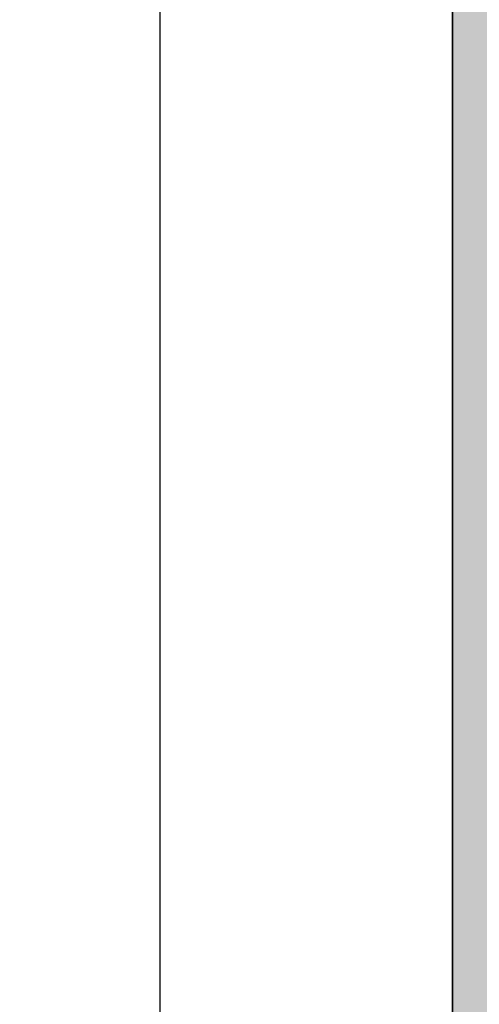
# Model space of a CAD drawing. Units: inches. Extents: x 3008 to 4088, y 1255 to 2137.
# Tile 14 of 30: x 3008 to 3042, y 1874 to 1945. Entities that reach past the tile are written whole.
import ezdxf

# ---------------------------------------------------------------- set-up
doc = ezdxf.new("R2010")
doc.units = ezdxf.units.IN
for name, color, linetype, lineweight in [('A-ANNO-DIMS', 2, 'Continuous', 18), ('C-PROP', 1, 'Continuous', 35), ('C-PROP-PATT', 9, 'Continuous', 13)]:
    doc.layers.add(name, color=color, linetype=linetype, lineweight=lineweight)
doc.styles.get("Standard").update_dxf_attribs({"font": 'arial.ttf'})
doc.dimstyles.new('ISO-25', dxfattribs={"dimtxt": 8, "dimasz": 2.5, "dimexe": 1.25, "dimexo": 0.625, "dimtad": 1, "dimdec": 1, "dimlunit": 3, "dimtxsty": 'Standard', "dimcen": 2.5, "dimadec": 0, "dimazin": 0, "dimtfac": 1, "dimtdec": 1, "dimtmove": 0, "dimatfit": 3, "dimfxl": 1, "dimarcsym": 0})

# ---------------------------------------------------------------- blocks, each defined once
blk = doc.blocks.new('*D2')
at = {"layer": 'A-ANNO-DIMS', "color": 0, "lineweight": -2, "transparency": 16777216}
for p, q in [((3039.041, 2003.966), (3017.26, 2003.966)), ((3018.51, 2001.466), (3018.51, 1346.466)), ((3039.041, 1343.966), (3017.26, 1343.966))]:
    blk.add_line(p, q, dxfattribs=at)
at = {"layer": 'A-ANNO-DIMS', "color": 0, "transparency": 16777216}
for points in [[(3018.093, 2001.466), (3018.927, 2001.466), (3018.51, 2003.966)], [(3018.093, 1346.466), (3018.927, 1346.466), (3018.51, 1343.966)]]:
    blk.add_solid(points, dxfattribs=at)
at = {"layer": 'Defpoints', "color": 0, "transparency": 16777216}
for p in [(3039.666, 2003.966), (3018.51, 1343.966), (3039.666, 1343.966)]:
    blk.add_point(p, dxfattribs=at)
at = {"layer": 'A-ANNO-DIMS', "color": 0, "transparency": 16777216, "insert": (3013.817, 1673.966), "char_height": 8, "attachment_point": 5, "rotation": 90}
blk.add_mtext("55'", dxfattribs=at)

msp = doc.modelspace()

# ---------------------------------------------------------------- hatches: boundary and pattern name
at = {"layer": 'C-PROP-PATT'}
h = msp.add_hatch(color=256, dxfattribs=at)
h.dxf.hatch_style = 1
h.paths.add_polyline_path([(3519.666, 2003.966), (3039.666, 2003.966), (3039.666, 1343.966), (3051.666, 1343.966), (3051.666, 1348.966), (3044.666, 1348.966), (3044.666, 1998.966), (3514.666, 1998.966), (3514.666, 1348.966), (3219.666, 1348.966), (3219.666, 1343.966), (3519.666, 1343.966)])

# ---------------------------------------------------------------- linework, layer by layer
at = {"layer": 'C-PROP'}
msp.add_line((3039.666, 1343.966), (3039.666, 2003.966), dxfattribs=at)

# ---------------------------------------------------------------- dimensions: what is measured, and where the dimension line sits
at = {"layer": 'A-ANNO-DIMS'}
dim = msp.add_linear_dim(base=(3018.51, 1343.966), p1=(3039.666, 2003.966), p2=(3039.666, 1343.966), angle=90, dimstyle='ISO-25', override={"dimclrd": 0, "dimclre": 0, "dimclrt": 0}, dxfattribs=at)
dim.commit()
dim.dimension.update_dxf_attribs({"geometry": '*D2', "text_midpoint": (3013.817, 1673.966)})

doc.saveas('drawing.dxf')
